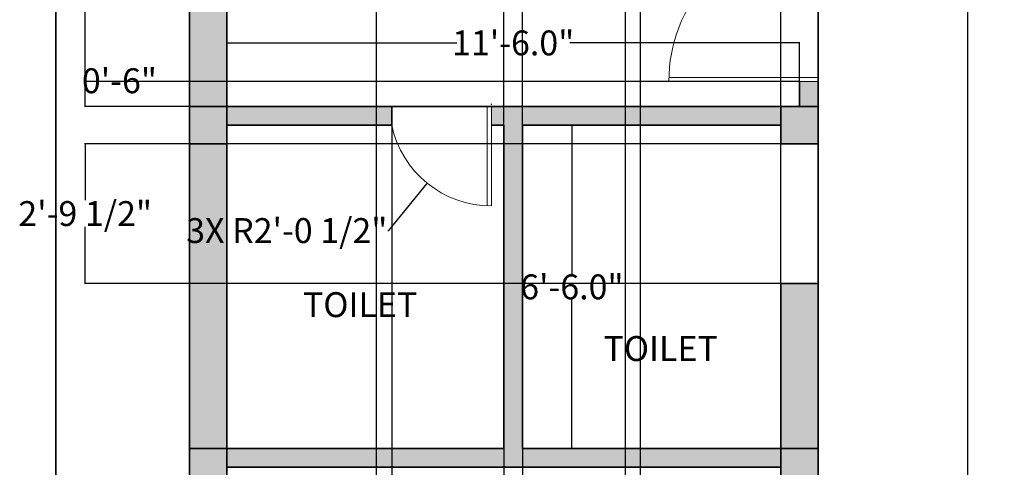
# Model space of a CAD drawing. Units: inches. Extents: x 74 to 548, y 68 to 649.
# Tile 4 of 6: x 74 to 311, y 361 to 469. Entities that reach past the tile are written whole.
import ezdxf

# ---------------------------------------------------------------- set-up
doc = ezdxf.new("R2010")
doc.units = ezdxf.units.IN
doc.header["$MEASUREMENT"] = 0
for name, color, linetype, lineweight in [('A-ANNO-DIMS', 2, 'Continuous', 18), ('A-ANNO-TTLB', 7, 'Continuous', 35), ('A-AREA-IDEN', 7, 'Continuous', 25), ('A-COLS', 7, 'Continuous', 35), ('A-DOOR', 3, 'Continuous', 18), ('A-WALL', 7, 'Continuous', 35)]:
    doc.layers.add(name, color=color, linetype=linetype, lineweight=lineweight)
doc.layers.add('A-COLS-PATT', color=11, linetype='Continuous', lineweight=13, true_color=0xf27172)
doc.layers.add('A-WALL-PATT', color=7, linetype='Continuous', lineweight=13, true_color=0xffffff)
doc.styles.get("Standard").update_dxf_attribs({"font": 'arial.ttf'})
doc.dimstyles.get("Standard").update_dxf_attribs({"dimtxt": 6, "dimasz": 0.18, "dimexe": 0.18, "dimexo": 0.0625, "dimgap": 0.09, "dimtad": 0, "dimtih": 1, "dimtoh": 1, "dimdec": 1, "dimzin": 0, "dimdsep": 46, "dimlunit": 3, "dimtxsty": 'Standard', "dimcen": 0.09, "dimadec": 0, "dimazin": 0, "dimtfac": 1, "dimtdec": 1, "dimtofl": 0, "dimtmove": 0, "dimatfit": 3, "dimfxl": 1, "dimtolj": 1, "dimtzin": 0, "dimarcsym": 0})

# ---------------------------------------------------------------- blocks, each defined once
blk = doc.blocks.new('*D6')
at = {"layer": 'A-ANNO-DIMS', "color": 0, "lineweight": -2, "transparency": 16777216}
for p, q in [((123.96, 457), (123.96, 463.72)), ((124.14, 463.54), (179.35, 463.54)), ((261.78, 463.54), (206.57, 463.54)), ((261.96, 451.31), (261.96, 463.72))]:
    blk.add_line(p, q, dxfattribs=at)
at = {"layer": 'A-ANNO-DIMS', "color": 0, "transparency": 16777216}
for points in [[(124.14, 463.57), (124.14, 463.51), (123.96, 463.54)], [(261.78, 463.57), (261.78, 463.51), (261.96, 463.54)]]:
    blk.add_solid(points, dxfattribs=at)
at = {"layer": 'Defpoints', "color": 0, "transparency": 16777216}
for p in [(261.96, 463.54), (123.96, 456.93), (261.96, 451.24)]:
    blk.add_point(p, dxfattribs=at)
at = {"layer": 'A-ANNO-DIMS', "color": 0, "transparency": 16777216, "insert": (192.96, 463.54), "char_height": 6, "attachment_point": 5}
blk.add_mtext('\\A1;11\'-6.0"', dxfattribs=at)
blk = doc.blocks.new('*D8')
at = {"layer": 'A-ANNO-DIMS', "color": 0, "lineweight": -2, "transparency": 16777216}
for p, q in [((203.64, 443.74), (207.28, 443.74)), ((207.1, 443.56), (207.1, 407.9)), ((207.1, 365.92), (207.1, 401.59)), ((203.64, 365.74), (207.28, 365.74))]:
    blk.add_line(p, q, dxfattribs=at)
at = {"layer": 'A-ANNO-DIMS', "color": 0, "transparency": 16777216}
for points in [[(207.07, 443.56), (207.13, 443.56), (207.1, 443.74)], [(207.07, 365.92), (207.13, 365.92), (207.1, 365.74)]]:
    blk.add_solid(points, dxfattribs=at)
at = {"layer": 'Defpoints', "color": 0, "transparency": 16777216}
for p in [(203.58, 443.74), (203.58, 365.74), (207.1, 365.74)]:
    blk.add_point(p, dxfattribs=at)
at = {"layer": 'A-ANNO-DIMS', "color": 0, "transparency": 16777216, "insert": (207.1, 404.74), "char_height": 6, "attachment_point": 5}
blk.add_mtext('\\A1;6\'-6.0"', dxfattribs=at)
blk = doc.blocks.new('DOOR-SWING-36IN')
for p, q in [((0, 0), (0, 36)), ((-36, 1), (0, 1)), ((0, 0), (-36, 0))]:
    blk.add_line(p, q)
blk.add_arc((0.32, 0), 36.32, 97.6281, 180)
blk = doc.blocks.new('DOOR-SWING-24IN')
for p, q in [((0, 0), (-24, 0)), ((-1, -24), (-1, 0)), ((0, 0), (0, -24))]:
    blk.add_line(p, q)
blk.add_arc((0, 0.52), 24.52, 191.8123, 270)
blk = doc.blocks.new('*D18')
at = {"layer": 'A-ANNO-DIMS', "color": 0, "lineweight": -2, "transparency": 16777216}
for p, q in [((114.9, 575.24), (89.68, 575.24)), ((89.86, 575.06), (89.86, 514.9)), ((89.86, 448.42), (89.86, 508.59)), ((123.9, 448.24), (89.68, 448.24))]:
    blk.add_line(p, q, dxfattribs=at)
at = {"layer": 'A-ANNO-DIMS', "color": 0, "transparency": 16777216}
for points in [[(89.83, 575.06), (89.89, 575.06), (89.86, 575.24)], [(89.83, 448.42), (89.89, 448.42), (89.86, 448.24)]]:
    blk.add_solid(points, dxfattribs=at)
at = {"layer": 'Defpoints', "color": 0, "transparency": 16777216}
for p in [(89.86, 575.24), (114.96, 575.24), (123.96, 448.24)]:
    blk.add_point(p, dxfattribs=at)
at = {"layer": 'A-ANNO-DIMS', "color": 0, "transparency": 16777216, "insert": (89.86, 511.74), "char_height": 6, "attachment_point": 5}
blk.add_mtext('\\A1;10\'-7"', dxfattribs=at)
blk = doc.blocks.new('*D19')
at = {"layer": 'A-ANNO-DIMS', "color": 0, "lineweight": -2, "transparency": 16777216}
for p, q in [((123.96, 361.31), (123.96, 609.52)), ((124.14, 609.34), (149.27, 609.34)), ((190.53, 609.34), (165.4, 609.34)), ((190.71, 365.81), (190.71, 609.52))]:
    blk.add_line(p, q, dxfattribs=at)
at = {"layer": 'A-ANNO-DIMS', "color": 0, "transparency": 16777216}
for points in [[(124.14, 609.37), (124.14, 609.31), (123.96, 609.34)], [(190.53, 609.37), (190.53, 609.31), (190.71, 609.34)]]:
    blk.add_solid(points, dxfattribs=at)
at = {"layer": 'Defpoints', "color": 0, "transparency": 16777216}
for p in [(190.71, 609.34), (190.71, 365.74), (123.96, 361.24)]:
    blk.add_point(p, dxfattribs=at)
at = {"layer": 'A-ANNO-DIMS', "color": 0, "transparency": 16777216, "insert": (157.34, 609.34), "char_height": 6, "attachment_point": 5}
blk.add_mtext('\\A1;5\'-7"', dxfattribs=at)
blk = doc.blocks.new('*D20')
at = {"layer": 'A-ANNO-DIMS', "color": 0, "lineweight": -2, "transparency": 16777216}
for p, q in [((195.21, 365.81), (195.21, 609.52)), ((195.39, 609.34), (211.28, 609.34)), ((257.28, 609.34), (241.39, 609.34)), ((257.46, 365.81), (257.46, 609.52))]:
    blk.add_line(p, q, dxfattribs=at)
at = {"layer": 'A-ANNO-DIMS', "color": 0, "transparency": 16777216}
for points in [[(195.39, 609.37), (195.39, 609.31), (195.21, 609.34)], [(257.28, 609.37), (257.28, 609.31), (257.46, 609.34)]]:
    blk.add_solid(points, dxfattribs=at)
at = {"layer": 'Defpoints', "color": 0, "transparency": 16777216}
for p in [(257.46, 609.34), (195.21, 365.74), (257.46, 365.74)]:
    blk.add_point(p, dxfattribs=at)
at = {"layer": 'A-ANNO-DIMS', "color": 0, "transparency": 16777216, "insert": (226.34, 609.34), "char_height": 6, "attachment_point": 5}
blk.add_mtext('\\A1;5\'-2 1/2"', dxfattribs=at)
blk = doc.blocks.new('*D30')
at = {"layer": 'A-ANNO-DIMS', "color": 0, "lineweight": -2, "transparency": 16777216}
for p, q in [((160.05, 220.81), (160.05, 609.52)), ((160.23, 609.34), (181.98, 609.34)), ((219.87, 609.34), (198.11, 609.34)), ((220.05, 220.81), (220.05, 609.52))]:
    blk.add_line(p, q, dxfattribs=at)
at = {"layer": 'A-ANNO-DIMS', "color": 0, "transparency": 16777216}
for points in [[(160.23, 609.37), (160.23, 609.31), (160.05, 609.34)], [(219.87, 609.37), (219.87, 609.31), (220.05, 609.34)]]:
    blk.add_solid(points, dxfattribs=at)
at = {"layer": 'Defpoints', "color": 0, "transparency": 16777216}
for p in [(220.05, 609.34), (160.05, 220.74), (220.05, 220.74)]:
    blk.add_point(p, dxfattribs=at)
at = {"layer": 'A-ANNO-DIMS', "color": 0, "transparency": 16777216, "insert": (190.05, 609.34), "char_height": 6, "attachment_point": 5}
blk.add_mtext('\\A1;5\'-0"', dxfattribs=at)
blk = doc.blocks.new('*D35')
at = {"layer": 'A-ANNO-DIMS', "color": 0, "lineweight": -2, "transparency": 16777216}
for p, q in [((190.71, 365.68), (190.71, 87.96)), ((195.21, 365.68), (195.21, 87.96)), ((190.89, 88.14), (195.03, 88.14)), ((195.21, 88.14), (195.39, 88.14))]:
    blk.add_line(p, q, dxfattribs=at)
at = {"layer": 'A-ANNO-DIMS', "color": 0, "transparency": 16777216}
for points in [[(190.89, 88.17), (190.89, 88.11), (190.71, 88.14)], [(195.03, 88.17), (195.03, 88.11), (195.21, 88.14)]]:
    blk.add_solid(points, dxfattribs=at)
at = {"layer": 'Defpoints', "color": 0, "transparency": 16777216}
for p in [(190.71, 365.74), (195.21, 365.74), (195.21, 88.14)]:
    blk.add_point(p, dxfattribs=at)
at = {"layer": 'A-ANNO-DIMS', "color": 0, "transparency": 16777216, "insert": (210.45, 88.14), "char_height": 6, "attachment_point": 5}
blk.add_mtext('\\A1;0\'-4 1/2"', dxfattribs=at)
blk = doc.blocks.new('*D36')
at = {"layer": 'A-ANNO-DIMS', "color": 0, "lineweight": -2, "transparency": 16777216}
for p, q in [((266.46, 223.31), (266.46, 609.52)), ((266.64, 609.34), (276.4, 609.34)), ((302.28, 609.34), (292.52, 609.34)), ((302.46, 223.31), (302.46, 609.52))]:
    blk.add_line(p, q, dxfattribs=at)
at = {"layer": 'A-ANNO-DIMS', "color": 0, "transparency": 16777216}
for points in [[(266.64, 609.37), (266.64, 609.31), (266.46, 609.34)], [(302.28, 609.37), (302.28, 609.31), (302.46, 609.34)]]:
    blk.add_solid(points, dxfattribs=at)
at = {"layer": 'Defpoints', "color": 0, "transparency": 16777216}
for p in [(302.46, 609.34), (266.46, 223.24), (302.46, 223.24)]:
    blk.add_point(p, dxfattribs=at)
at = {"layer": 'A-ANNO-DIMS', "color": 0, "transparency": 16777216, "insert": (284.46, 609.34), "char_height": 6, "attachment_point": 5}
blk.add_mtext('\\A1;3\'-0"', dxfattribs=at)
blk = doc.blocks.new('*D37')
at = {"layer": 'A-ANNO-DIMS', "color": 0, "lineweight": -2, "transparency": 16777216}
for p, q in [((266.46, 297.87), (266.46, 609.52)), ((266.64, 609.34), (322.83, 609.34)), ((399.25, 609.34), (343.06, 609.34)), ((399.43, 299.06), (399.43, 609.52))]:
    blk.add_line(p, q, dxfattribs=at)
at = {"layer": 'A-ANNO-DIMS', "color": 0, "transparency": 16777216}
for points in [[(266.64, 609.37), (266.64, 609.31), (266.46, 609.34)], [(399.25, 609.37), (399.25, 609.31), (399.43, 609.34)]]:
    blk.add_solid(points, dxfattribs=at)
at = {"layer": 'Defpoints', "color": 0, "transparency": 16777216}
for p in [(399.43, 609.34), (399.43, 298.99), (266.46, 297.81)]:
    blk.add_point(p, dxfattribs=at)
at = {"layer": 'A-ANNO-DIMS', "color": 0, "transparency": 16777216, "insert": (332.94, 609.34), "char_height": 6, "attachment_point": 5}
blk.add_mtext('\\A1;11\'-1"', dxfattribs=at)
blk = doc.blocks.new('*D40')
at = {"layer": 'A-ANNO-DIMS', "color": 0, "lineweight": -2, "transparency": 16777216}
for p, q in [((266.4, 439.24), (89.68, 439.24)), ((89.86, 439.06), (89.86, 425.6)), ((89.86, 405.76), (89.86, 419.22)), ((266.4, 405.58), (89.68, 405.58))]:
    blk.add_line(p, q, dxfattribs=at)
at = {"layer": 'A-ANNO-DIMS', "color": 0, "transparency": 16777216}
for points in [[(89.83, 439.06), (89.89, 439.06), (89.86, 439.24)], [(89.83, 405.76), (89.89, 405.76), (89.86, 405.58)]]:
    blk.add_solid(points, dxfattribs=at)
at = {"layer": 'Defpoints', "color": 0, "transparency": 16777216}
for p in [(89.86, 439.24), (266.46, 439.24), (266.46, 405.58)]:
    blk.add_point(p, dxfattribs=at)
at = {"layer": 'A-ANNO-DIMS', "color": 0, "transparency": 16777216, "insert": (89.86, 422.41), "char_height": 6, "attachment_point": 5}
blk.add_mtext('\\A1;2\'-9 1/2"', dxfattribs=at)
blk = doc.blocks.new('*D42')
at = {"layer": 'A-ANNO-DIMS', "color": 0, "lineweight": -2, "transparency": 16777216}
for p, q in [((223.59, 223.31), (223.59, 609.52)), ((223.77, 609.34), (230.08, 609.34)), ((257.28, 609.34), (250.97, 609.34)), ((257.46, 223.31), (257.46, 609.52))]:
    blk.add_line(p, q, dxfattribs=at)
at = {"layer": 'A-ANNO-DIMS', "color": 0, "transparency": 16777216}
for points in [[(223.77, 609.37), (223.77, 609.31), (223.59, 609.34)], [(257.28, 609.37), (257.28, 609.31), (257.46, 609.34)]]:
    blk.add_solid(points, dxfattribs=at)
at = {"layer": 'Defpoints', "color": 0, "transparency": 16777216}
for p in [(257.46, 609.34), (223.59, 223.24), (257.46, 223.24)]:
    blk.add_point(p, dxfattribs=at)
at = {"layer": 'A-ANNO-DIMS', "color": 0, "transparency": 16777216, "insert": (240.52, 609.34), "char_height": 6, "attachment_point": 5}
blk.add_mtext('\\A1;2\'-10"', dxfattribs=at)
blk = doc.blocks.new('*D43')
at = {"layer": 'A-ANNO-DIMS', "color": 0, "lineweight": -2, "transparency": 16777216}
for p, q in [((261.9, 454.24), (89.68, 454.24)), ((89.86, 454.24), (89.86, 454.42)), ((89.86, 454.42), (90.04, 454.42)), ((89.86, 448.42), (89.86, 454.06)), ((257.4, 448.24), (89.68, 448.24))]:
    blk.add_line(p, q, dxfattribs=at)
at = {"layer": 'A-ANNO-DIMS', "color": 0, "transparency": 16777216}
for points in [[(89.83, 454.06), (89.89, 454.06), (89.86, 454.24)], [(89.83, 448.42), (89.89, 448.42), (89.86, 448.24)]]:
    blk.add_solid(points, dxfattribs=at)
at = {"layer": 'Defpoints', "color": 0, "transparency": 16777216}
for p in [(89.86, 454.24), (261.96, 454.24), (257.46, 448.24)]:
    blk.add_point(p, dxfattribs=at)
at = {"layer": 'A-ANNO-DIMS', "color": 0, "transparency": 16777216, "insert": (98.11, 454.42), "char_height": 6, "attachment_point": 5}
blk.add_mtext('\\A1;0\'-6"', dxfattribs=at)
blk = doc.blocks.new('*D44')
at = {"layer": 'A-ANNO-DIMS', "color": 0, "lineweight": -2, "transparency": 16777216}
for p, q in [((163.71, 448.18), (163.71, 87.96)), ((123.96, 439.18), (123.96, 87.96)), ((124.14, 88.14), (135.77, 88.14)), ((163.53, 88.14), (151.9, 88.14))]:
    blk.add_line(p, q, dxfattribs=at)
at = {"layer": 'A-ANNO-DIMS', "color": 0, "transparency": 16777216}
for points in [[(124.14, 88.17), (124.14, 88.11), (123.96, 88.14)], [(163.53, 88.17), (163.53, 88.11), (163.71, 88.14)]]:
    blk.add_solid(points, dxfattribs=at)
at = {"layer": 'Defpoints', "color": 0, "transparency": 16777216}
for p in [(163.71, 448.24), (123.96, 439.24), (163.71, 88.14)]:
    blk.add_point(p, dxfattribs=at)
at = {"layer": 'A-ANNO-DIMS', "color": 0, "transparency": 16777216, "insert": (143.84, 88.14), "char_height": 6, "attachment_point": 5}
blk.add_mtext('\\A1;3\'-4"', dxfattribs=at)
blk = doc.blocks.new('*D45')
at = {"layer": 'A-ANNO-DIMS', "color": 0, "lineweight": -2, "transparency": 16777216}
for p, q in [((187.62, 448.76), (187.8, 448.76)), ((187.71, 448.67), (187.71, 448.85)), ((162.97, 418.31), (172.14, 429.59)), ((162.79, 418.31), (162.97, 418.31))]:
    blk.add_line(p, q, dxfattribs=at)
at = {"layer": 'A-ANNO-DIMS', "color": 0, "transparency": 16777216}
blk.add_solid([(172.11, 429.61), (172.16, 429.57), (172.25, 429.73)], dxfattribs=at)
at = {"layer": 'Defpoints', "color": 0, "transparency": 16777216}
for p in [(187.71, 448.76), (172.25, 429.73)]:
    blk.add_point(p, dxfattribs=at)
at = {"layer": 'A-ANNO-DIMS', "color": 0, "transparency": 16777216, "insert": (138.42, 418.31), "char_height": 6, "attachment_point": 5}
blk.add_mtext('\\A1;3X R2\'-0 1/2"', dxfattribs=at)

msp = doc.modelspace()

# ---------------------------------------------------------------- hatches: boundary and pattern name
at = {"layer": 'A-COLS-PATT'}
h = msp.add_hatch(color=256, dxfattribs=at)
h.dxf.hatch_style = 1
h.paths.add_polyline_path([(123.96, 584.24), (114.96, 584.24), (114.96, 575.24), (123.96, 575.24)])
h.paths.add_polyline_path([(266.46, 584.24), (257.46, 584.24), (257.46, 575.24), (266.46, 575.24)])
h.paths.add_polyline_path([(329.46, 584.24), (320.46, 584.24), (320.46, 575.24), (329.46, 575.24)])
h.paths.add_polyline_path([(471.96, 584.24), (462.96, 584.24), (462.96, 575.24), (471.96, 575.24)])
h.paths.add_polyline_path([(123.96, 448.24), (114.96, 448.24), (114.96, 439.24), (123.96, 439.24)])
h.paths.add_polyline_path([(266.46, 448.24), (261.96, 448.24), (257.46, 448.24), (257.46, 439.24), (266.46, 439.24)])
h.paths.add_polyline_path([(329.46, 448.24), (320.46, 448.24), (320.46, 439.24), (329.46, 439.24)])
h.paths.add_polyline_path([(471.96, 448.24), (462.96, 448.24), (462.96, 439.24), (471.96, 439.24)])
h.paths.add_polyline_path([(123.96, 365.74), (114.96, 365.74), (114.96, 356.74), (123.96, 356.74)])
h.paths.add_polyline_path([(266.46, 365.74), (257.46, 365.74), (257.46, 356.74), (266.46, 356.74)])
h.paths.add_polyline_path([(123.96, 223.24), (114.96, 223.24), (114.96, 214.24), (123.96, 214.24)])
h.paths.add_polyline_path([(266.46, 223.24), (257.46, 223.24), (257.46, 214.24), (266.46, 214.24)])
h.paths.add_polyline_path([(123.96, 142.24), (114.96, 142.24), (114.96, 133.24), (123.96, 133.24)])
h.paths.add_polyline_path([(263.89, 142.24), (254.89, 142.24), (254.89, 133.24), (263.89, 133.24)])
h.paths.add_polyline_path([(471.96, 142.24), (462.96, 142.24), (462.96, 133.24), (471.96, 133.24)])
h.paths.add_polyline_path([(377.46, 142.24), (368.46, 142.24), (368.46, 133.24), (377.46, 133.24)])
h.paths.add_polyline_path([(377.46, 223.24), (368.46, 223.24), (368.46, 214.24), (377.46, 214.24)])
h.paths.add_polyline_path([(471.96, 223.24), (462.96, 223.24), (462.96, 214.24), (471.96, 214.24)])
h.paths.add_polyline_path([(471.96, 298.99), (462.96, 298.99), (462.96, 289.99), (471.96, 289.99)])
h.paths.add_polyline_path([(471.96, 365.74), (462.96, 365.74), (462.96, 356.74), (471.96, 356.74)])
at = {"layer": 'A-WALL-PATT'}
h = msp.add_hatch(color=256, dxfattribs=at)
h.dxf.hatch_style = 1
h.paths.add_polyline_path([(123.96, 356.74), (114.96, 356.74), (114.96, 223.24), (123.96, 223.24)])
h.paths.add_polyline_path([(123.96, 439.24), (114.96, 439.24), (114.96, 365.74), (123.96, 365.74)])
h.paths.add_polyline_path([(123.96, 575.24), (114.96, 575.24), (114.96, 448.24), (123.96, 448.24)])
h.paths.add_polyline_path([(257.46, 584.24), (123.96, 584.24), (123.96, 575.24), (257.46, 575.24)])
h.paths.add_polyline_path([(266.46, 575.24), (261.96, 575.24), (261.96, 490.24), (266.46, 490.24)])
h.paths.add_polyline_path([(266.46, 454.24), (261.96, 454.24), (261.96, 448.24), (266.46, 448.24)])
h.paths.add_polyline_path([(257.46, 448.24), (187.71, 448.24), (187.71, 443.74), (190.71, 443.74), (190.71, 365.74), (123.96, 365.74), (123.96, 361.24), (257.46, 361.24), (257.46, 365.74), (195.21, 365.74), (195.21, 443.74), (257.46, 443.74)])
h.paths.add_polyline_path([(163.71, 448.24), (123.96, 448.24), (123.96, 443.74), (163.71, 443.74)], flags=17)
h.paths.add_polyline_path([(223.59, 223.24), (220.05, 223.24), (220.05, 216.24), (160.05, 216.24), (160.05, 223.24), (123.96, 223.24), (123.96, 214.24), (159.96, 214.24), (223.59, 214.24)])
h.paths.add_polyline_path([(123.96, 214.24), (114.96, 214.24), (114.96, 142.24), (123.96, 142.24)])
h.paths.add_polyline_path([(254.89, 142.24), (123.96, 142.24), (123.96, 133.24), (254.89, 133.24)])
h.paths.add_polyline_path([(462.96, 142.24), (377.46, 142.24), (377.46, 133.24), (462.96, 133.24)])
h.paths.add_polyline_path([(372.96, 189.24), (368.46, 189.24), (368.46, 142.24), (372.96, 142.24)])
h.paths.add_polyline_path([(471.96, 214.24), (462.96, 214.24), (462.96, 142.24), (471.96, 142.24)])
h.paths.add_polyline_path([(462.96, 223.24), (403.93, 223.24), (403.93, 294.49), (409.93, 294.49), (409.93, 298.99), (403.93, 298.99), (399.43, 298.99), (399.43, 223.24), (377.46, 223.24), (377.46, 214.24), (462.96, 214.24)])
h.paths.add_polyline_path([(368.46, 223.24), (353.46, 223.24), (353.46, 216.24), (305.46, 216.24), (305.46, 223.24), (302.46, 223.24), (302.46, 214.24), (368.46, 214.24)])
h.paths.add_polyline_path([(471.96, 289.99), (462.96, 289.99), (462.96, 223.24), (471.96, 223.24)])
h.paths.add_polyline_path([(462.96, 298.99), (433.93, 298.99), (433.93, 294.49), (462.96, 294.49)], flags=0)
h.paths.add_polyline_path([(471.96, 356.74), (462.96, 356.74), (462.96, 298.99), (471.96, 298.99)])
h.paths.add_polyline_path([(462.96, 365.74), (403.93, 365.74), (403.93, 361.24), (462.96, 361.24)], flags=17)
h.paths.add_polyline_path([(471.96, 439.24), (462.96, 439.24), (462.96, 365.74), (471.96, 365.74)])
h.paths.add_polyline_path([(462.96, 448.24), (329.46, 448.24), (329.46, 439.24), (368.46, 439.24), (368.46, 361.24), (372.96, 361.24), (372.96, 443.74), (462.96, 443.74)])
h.paths.add_polyline_path([(324.96, 454.24), (320.46, 454.24), (320.46, 448.24), (324.96, 448.24)])
h.paths.add_polyline_path([(471.96, 575.24), (462.96, 575.24), (462.96, 448.24), (471.96, 448.24)])
h.paths.add_polyline_path([(462.96, 584.24), (329.46, 584.24), (329.46, 575.24), (462.96, 575.24)])
h.paths.add_polyline_path([(320.46, 584.24), (266.46, 584.24), (266.46, 575.24), (320.46, 575.24)])
h.paths.add_polyline_path([(324.96, 575.24), (320.46, 575.24), (320.46, 490.24), (324.96, 490.24)])
h.paths.add_polyline_path([(266.46, 405.58), (257.46, 405.58), (257.46, 365.74), (266.46, 365.74)])
h.paths.add_polyline_path([(266.46, 356.74), (261.96, 356.74), (261.96, 333.81), (266.46, 333.81)])
h.paths.add_polyline_path([(266.46, 297.81), (261.96, 297.81), (261.96, 223.24), (266.46, 223.24)])

# ---------------------------------------------------------------- linework, layer by layer
at = {"layer": 'A-ANNO-TTLB'}
msp.add_lwpolyline([(82.75, 649.38), (548.44, 649.38), (548.44, 68.13), (82.75, 68.13)], close=True, dxfattribs=at)
at = {"layer": 'A-COLS'}
for p, q in [((123.96, 448.24), (114.96, 448.24)), ((114.96, 448.24), (114.96, 439.24)), ((261.96, 448.24), (257.46, 448.24)), ((257.46, 448.24), (257.46, 439.24)), ((261.96, 448.24), (266.46, 448.24)), ((114.96, 439.24), (123.96, 439.24)), ((257.46, 439.24), (266.46, 439.24)), ((257.46, 365.74), (257.46, 356.74))]:
    msp.add_line(p, q, dxfattribs=at)
at = {"layer": 'A-DOOR'}
for p, q in [((230.46, 454.24), (266.46, 454.24)), ((187.71, 424.24), (187.71, 448.24))]:
    msp.add_line(p, q, dxfattribs=at)
at = {"layer": 'A-WALL'}
for p, q in [((114.96, 584.24), (114.96, 133.24)), ((123.96, 584.24), (123.96, 133.24)), ((266.46, 584.24), (266.46, 214.24)), ((261.96, 454.24), (261.96, 448.24)), ((266.46, 448.24), (266.46, 454.24)), ((123.96, 448.24), (257.46, 448.24)), ((163.71, 448.24), (163.71, 443.74)), ((190.71, 448.24), (187.71, 448.24)), ((123.96, 443.74), (163.71, 443.74)), ((187.71, 443.74), (190.71, 443.74)), ((190.71, 365.74), (190.71, 443.74)), ((195.21, 365.74), (195.21, 443.74)), ((195.21, 443.74), (257.46, 443.74)), ((257.46, 405.58), (257.46, 365.74)), ((257.46, 405.58), (266.46, 405.58)), ((114.96, 365.74), (190.71, 365.74)), ((195.21, 365.74), (266.46, 365.74)), ((123.96, 361.24), (257.46, 361.24))]:
    msp.add_line(p, q, dxfattribs=at)

# ---------------------------------------------------------------- block references
at = {"layer": 'A-DOOR'}
for name, p in [('DOOR-SWING-36IN', (266.46, 454.24)), ('DOOR-SWING-24IN', (187.71, 448.24))]:
    msp.add_blockref(name, p, dxfattribs=at)

# ---------------------------------------------------------------- texts
at = {"layer": 'A-AREA-IDEN', "char_height": 6, "attachment_point": 1}
for width, insert in [(31.9877, (142.31, 403.45)), (36.0808, (214.71, 392.87))]:
    msp.add_mtext_dynamic_manual_height_columns('TOILET', width=width, gutter_width=30, heights=[0], dxfattribs=dict(at, insert=insert))

# ---------------------------------------------------------------- dimensions: what is measured, and where the dimension line sits
at = {"layer": 'A-ANNO-DIMS'}
for base, p1, p2, override, picture, middle in [((257.460646, 609.342592), (195.210646, 365.742592), (257.460646, 365.742592), {"dimdec": 1, "dimlfac": 1, "dimrnd": 0, "dimzin": 1, "dimdsep": 46, "dimlunit": 4, "dimfrac": 2}, '*D20', (226.335646, 609.342592)), ((190.710646, 609.342592), (123.960646, 361.242592), (190.710646, 365.742592), {"dimdec": 1, "dimlfac": 1, "dimrnd": 0, "dimzin": 1, "dimdsep": 46, "dimlunit": 4, "dimfrac": 2}, '*D19', (157.335646, 609.342592)), ((220.05, 609.34), (160.05, 220.74), (220.05, 220.74), {"dimdec": 1, "dimlfac": 1, "dimrnd": 0, "dimzin": 1, "dimdsep": 46, "dimlunit": 4, "dimfrac": 2}, '*D30', (190.05, 609.34)), ((257.46, 609.34), (223.59, 223.24), (257.46, 223.24), {"dimdec": 1, "dimlfac": 1, "dimrnd": 0, "dimzin": 1, "dimdsep": 46, "dimlunit": 4, "dimfrac": 2}, '*D42', (240.52, 609.34)), ((302.46, 609.34), (266.46, 223.24), (302.46, 223.24), {"dimdec": 1, "dimlfac": 1, "dimrnd": 0, "dimzin": 1, "dimdsep": 46, "dimlunit": 4, "dimfrac": 2}, '*D36', (284.46, 609.34)), ((399.43, 609.34), (266.46, 297.81), (399.43, 298.99), {"dimdec": 1, "dimlfac": 1, "dimrnd": 0, "dimzin": 1, "dimdsep": 46, "dimlunit": 4, "dimfrac": 2}, '*D37', (332.94, 609.34)), ((261.96, 463.54), (123.96, 456.93), (261.96, 451.24), {"dimclrd": 0, "dimclre": 0, "dimclrt": 0}, '*D6', (192.96, 463.54)), ((163.710646, 88.142592), (123.960646, 439.242592), (163.710646, 448.242592), {"dimdec": 1, "dimlfac": 1, "dimrnd": 0, "dimzin": 1, "dimdsep": 46, "dimlunit": 4, "dimfrac": 2}, '*D44', (143.835646, 88.142592)), ((195.21, 88.14), (190.71, 365.74), (195.21, 365.74), {"dimdec": 1, "dimlfac": 1, "dimrnd": 0, "dimzin": 1, "dimdsep": 46, "dimlunit": 4, "dimfrac": 2}, '*D35', (210.45, 88.14))]:
    dim = msp.add_linear_dim(base=base, p1=p1, p2=p2, dimstyle='Standard', override=override, dxfattribs=at)
    dim.commit()
    dim.dimension.update_dxf_attribs({"geometry": picture, "text_midpoint": middle})
for base, p1, p2, override, picture, middle in [((89.86, 575.24), (123.96, 448.24), (114.96, 575.24), {"dimdec": 1, "dimlfac": 1, "dimrnd": 0, "dimzin": 1, "dimdsep": 46, "dimlunit": 4, "dimfrac": 2}, '*D18', (89.86, 511.74)), ((89.86, 454.24), (257.46, 448.24), (261.96, 454.24), {"dimdec": 1, "dimlfac": 1, "dimrnd": 0, "dimzin": 1, "dimdsep": 46, "dimlunit": 4, "dimfrac": 2}, '*D43', (98.11, 454.42)), ((207.1, 365.74), (203.58, 443.74), (203.58, 365.74), {"dimclrd": 0, "dimclre": 0, "dimclrt": 0}, '*D8', (207.1, 404.74)), ((89.86, 439.24), (266.46, 405.58), (266.46, 439.24), {"dimdec": 1, "dimlfac": 1, "dimrnd": 0, "dimzin": 1, "dimdsep": 46, "dimlunit": 4, "dimfrac": 2}, '*D40', (89.86, 422.41))]:
    dim = msp.add_linear_dim(base=base, p1=p1, p2=p2, angle=90, dimstyle='Standard', override=override, dxfattribs=at)
    dim.commit()
    dim.dimension.update_dxf_attribs({"geometry": picture, "text_midpoint": middle})
dim = msp.add_radius_dim(center=(187.71, 448.76), mpoint=(172.25, 429.73), text='3X <>', dimstyle='Standard', override={"dimdec": 1, "dimlfac": 1, "dimrnd": 0, "dimzin": 1, "dimdsep": 46, "dimlunit": 4, "dimfrac": 2}, dxfattribs=at)
dim.commit()
dim.dimension.update_dxf_attribs({"geometry": '*D45', "text_midpoint": (138.42, 418.31), "dimtype": 164})

doc.saveas('drawing.dxf')
